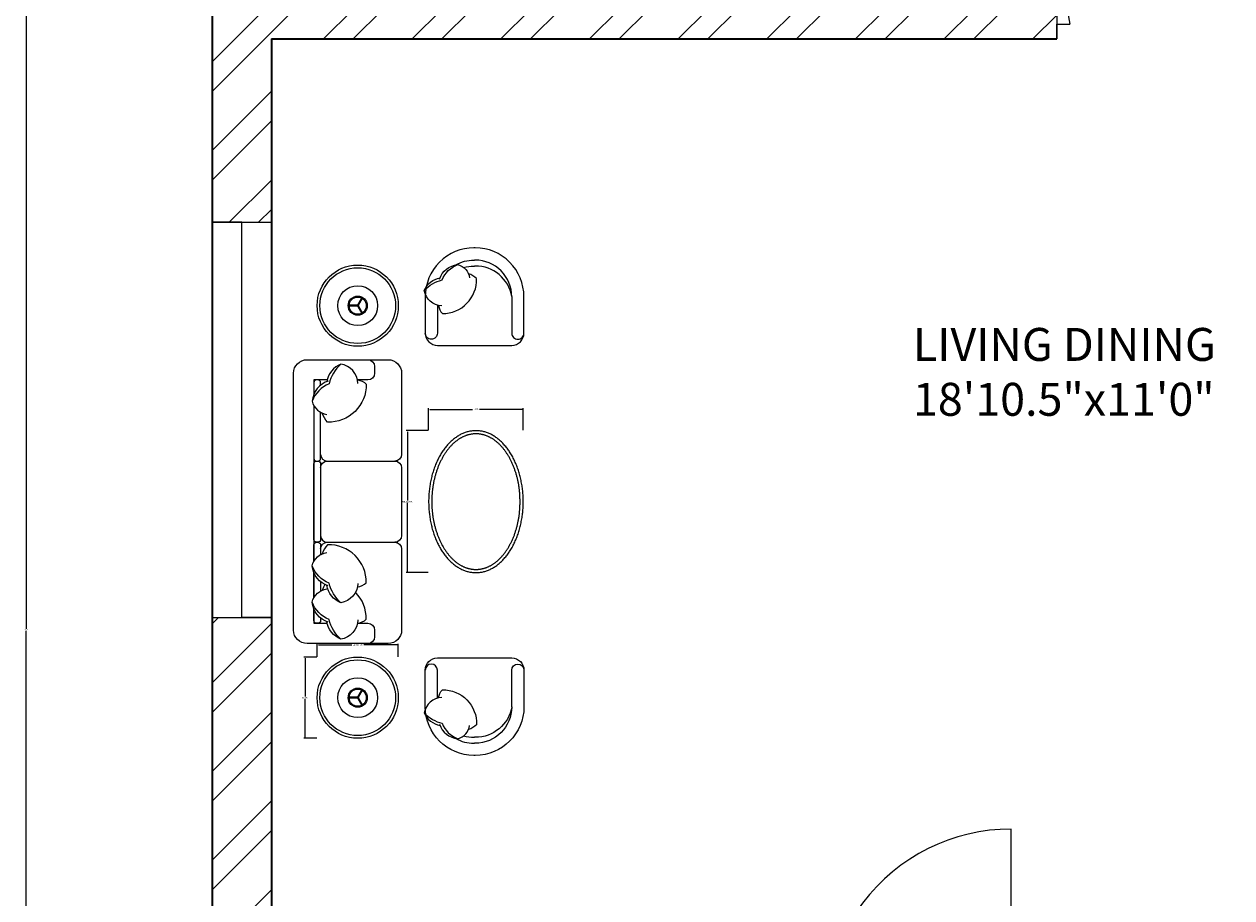
# Model space of a CAD drawing. Units: inches. Extents: x 1850 to 3445, y 1558 to 2756.
# Tile 2 of 13: x 2012 to 2195, y 1940 to 2073. Entities that reach past the tile are written whole.
import ezdxf

# ---------------------------------------------------------------- set-up
doc = ezdxf.new("R2010")
doc.units = ezdxf.units.IN
for name, color, linetype, lineweight in [('A-ANNO-DIMS', 2, 'Continuous', 18), ('A-AREA-IDEN', 7, 'Continuous', 18), ('A-DOOR', 3, 'Continuous', 18), ('A-FURN', 8, 'Continuous', 13), ('A-GLAZ', 4, 'Continuous', 18), ('A-WALL', 7, 'Continuous', 35), ('A-WALL-PATT', 252, 'Continuous', 13)]:
    doc.layers.add(name, color=color, linetype=linetype, lineweight=lineweight)
doc.styles.get("Standard").update_dxf_attribs({"font": 'arial.ttf'})
doc.dimstyles.get("Standard").update_dxf_attribs({"dimtxt": 0.18, "dimasz": 0.18, "dimexe": 0.18, "dimexo": 0.0625, "dimgap": 0.09, "dimtad": 0, "dimtih": 1, "dimtoh": 1, "dimdec": 4, "dimzin": 0, "dimdsep": 46, "dimtxsty": 'Standard', "dimcen": 0.09, "dimadec": 0, "dimazin": 0, "dimtfac": 1, "dimtdec": 4, "dimtofl": 0, "dimtmove": 0, "dimatfit": 3, "dimfxl": 1, "dimtolj": 1, "dimtzin": 0, "dimarcsym": 0})

# ---------------------------------------------------------------- blocks, each defined once
blk = doc.blocks.new('LAMP-ROUND-PLAN')
at = {"ltscale": 0.03}
for p, q in [((6.1, 6.13), (5.38, 7.38)), ((6.21, 6.19), (5.49, 7.44)), ((6.1, 6.19), (5.38, 4.94)), ((6.21, 6.13), (5.49, 4.87)), ((6.16, 6.22), (7.61, 6.22)), ((6.16, 6.09), (7.61, 6.09))]:
    blk.add_line(p, q, dxfattribs=at)
for radius in [6.16, 3.03, 1.45, 1.3]:
    blk.add_circle((6.16, 6.16), radius, dxfattribs=at)
blk.add_circle((6.16, 6.16), 5.75)
blk = doc.blocks.new('TABLE-COFFEE-OVAL')
at = {"ltscale": 0.03}
blk.add_polyline3d([(7.18, 0, 0), (7.32, 0, 0), (7.46, 0.01, 0), (7.59, 0.02, 0), (7.73, 0.03, 0), (7.86, 0.05, 0), (8, 0.07, 0), (8.13, 0.09, 0), (8.27, 0.12, 0), (8.4, 0.16, 0), (8.54, 0.19, 0), (8.67, 0.23, 0), (8.8, 0.28, 0), (8.93, 0.32, 0), (9.07, 0.38, 0), (9.2, 0.43, 0), (9.33, 0.49, 0), (9.46, 0.55, 0), (9.58, 0.62, 0), (9.71, 0.69, 0), (9.84, 0.76, 0), (9.96, 0.84, 0), (10.09, 0.92, 0), (10.21, 1.01, 0), (10.34, 1.09, 0), (10.46, 1.18, 0), (10.58, 1.28, 0), (10.7, 1.38, 0), (10.82, 1.48, 0), (10.93, 1.58, 0), (11.05, 1.69, 0), (11.16, 1.8, 0), (11.27, 1.92, 0), (11.38, 2.03, 0), (11.49, 2.16, 0), (11.6, 2.28, 0), (11.71, 2.41, 0), (11.81, 2.54, 0), (11.92, 2.67, 0), (12.02, 2.8, 0), (12.12, 2.94, 0), (12.22, 3.08, 0), (12.31, 3.23, 0), (12.41, 3.38, 0), (12.5, 3.53, 0), (12.59, 3.68, 0), (12.68, 3.83, 0), (12.76, 3.99, 0), (12.85, 4.15, 0), (12.93, 4.31, 0), (13.01, 4.48, 0), (13.09, 4.64, 0), (13.17, 4.81, 0), (13.24, 4.98, 0), (13.31, 5.15, 0), (13.38, 5.33, 0), (13.45, 5.51, 0), (13.52, 5.69, 0), (13.58, 5.87, 0), (13.64, 6.05, 0), (13.7, 6.23, 0), (13.75, 6.42, 0), (13.81, 6.61, 0), (13.86, 6.79, 0), (13.91, 6.98, 0), (13.96, 7.18, 0), (14, 7.37, 0), (14.04, 7.56, 0), (14.08, 7.76, 0), (14.12, 7.95, 0), (14.15, 8.15, 0), (14.18, 8.35, 0), (14.21, 8.55, 0), (14.24, 8.75, 0), (14.26, 8.95, 0), (14.29, 9.15, 0), (14.31, 9.35, 0), (14.32, 9.56, 0), (14.34, 9.76, 0), (14.35, 9.96, 0), (14.36, 10.17, 0), (14.36, 10.37, 0), (14.37, 10.57, 0), (14.37, 10.78, 0), (14.37, 10.98, 0), (14.36, 11.18, 0), (14.36, 11.39, 0), (14.35, 11.59, 0), (14.34, 11.8, 0), (14.32, 12, 0), (14.31, 12.2, 0), (14.29, 12.4, 0), (14.26, 12.6, 0), (14.24, 12.8, 0), (14.21, 13, 0), (14.18, 13.2, 0), (14.15, 13.4, 0), (14.12, 13.6, 0), (14.08, 13.8, 0), (14.04, 13.99, 0), (14, 14.18, 0), (13.96, 14.38, 0), (13.91, 14.57, 0), (13.86, 14.76, 0), (13.81, 14.95, 0), (13.75, 15.14, 0), (13.7, 15.32, 0), (13.64, 15.5, 0), (13.58, 15.69, 0), (13.52, 15.87, 0), (13.45, 16.05, 0), (13.38, 16.22, 0), (13.31, 16.4, 0), (13.24, 16.57, 0), (13.17, 16.74, 0), (13.09, 16.91, 0), (13.01, 17.08, 0), (12.93, 17.24, 0), (12.85, 17.4, 0), (12.76, 17.56, 0), (12.68, 17.72, 0), (12.59, 17.88, 0), (12.5, 18.03, 0), (12.41, 18.18, 0), (12.31, 18.32, 0), (12.22, 18.47, 0), (12.12, 18.61, 0), (12.02, 18.75, 0), (11.92, 18.88, 0), (11.81, 19.02, 0), (11.71, 19.15, 0), (11.6, 19.27, 0), (11.49, 19.4, 0), (11.38, 19.52, 0), (11.27, 19.64, 0), (11.16, 19.75, 0), (11.05, 19.86, 0), (10.93, 19.97, 0), (10.82, 20.08, 0), (10.7, 20.18, 0), (10.58, 20.27, 0), (10.46, 20.37, 0), (10.34, 20.46, 0), (10.21, 20.55, 0), (10.09, 20.63, 0), (9.96, 20.71, 0), (9.84, 20.79, 0), (9.71, 20.86, 0), (9.58, 20.93, 0), (9.46, 21, 0), (9.33, 21.06, 0), (9.2, 21.12, 0), (9.07, 21.18, 0), (8.93, 21.23, 0), (8.8, 21.28, 0), (8.67, 21.32, 0), (8.54, 21.36, 0), (8.4, 21.4, 0), (8.27, 21.43, 0), (8.13, 21.46, 0), (8, 21.48, 0), (7.86, 21.5, 0), (7.73, 21.52, 0), (7.59, 21.54, 0), (7.46, 21.55, 0), (7.32, 21.55, 0), (7.18, 21.55, 0), (7.05, 21.55, 0), (6.91, 21.55, 0), (6.78, 21.54, 0), (6.64, 21.52, 0), (6.5, 21.5, 0), (6.37, 21.48, 0), (6.23, 21.46, 0), (6.1, 21.43, 0), (5.97, 21.4, 0), (5.83, 21.36, 0), (5.7, 21.32, 0), (5.57, 21.28, 0), (5.43, 21.23, 0), (5.3, 21.18, 0), (5.17, 21.12, 0), (5.04, 21.06, 0), (4.91, 21, 0), (4.78, 20.93, 0), (4.66, 20.86, 0), (4.53, 20.79, 0), (4.4, 20.71, 0), (4.28, 20.63, 0), (4.15, 20.55, 0), (4.03, 20.46, 0), (3.91, 20.37, 0), (3.79, 20.27, 0), (3.67, 20.18, 0), (3.55, 20.08, 0), (3.44, 19.97, 0), (3.32, 19.86, 0), (3.21, 19.75, 0), (3.09, 19.64, 0), (2.98, 19.52, 0), (2.87, 19.4, 0), (2.77, 19.27, 0), (2.66, 19.15, 0), (2.55, 19.02, 0), (2.45, 18.88, 0), (2.35, 18.75, 0), (2.25, 18.61, 0), (2.15, 18.47, 0), (2.06, 18.32, 0), (1.96, 18.18, 0), (1.87, 18.03, 0), (1.78, 17.88, 0), (1.69, 17.72, 0), (1.6, 17.56, 0), (1.52, 17.4, 0), (1.44, 17.24, 0), (1.36, 17.08, 0), (1.28, 16.91, 0), (1.2, 16.74, 0), (1.13, 16.57, 0), (1.05, 16.4, 0), (0.98, 16.22, 0), (0.92, 16.05, 0), (0.85, 15.87, 0), (0.79, 15.69, 0), (0.73, 15.5, 0), (0.67, 15.32, 0), (0.61, 15.14, 0), (0.56, 14.95, 0), (0.51, 14.76, 0), (0.46, 14.57, 0), (0.41, 14.38, 0), (0.37, 14.18, 0), (0.33, 13.99, 0), (0.29, 13.8, 0), (0.25, 13.6, 0), (0.22, 13.4, 0), (0.18, 13.2, 0), (0.15, 13, 0), (0.13, 12.8, 0), (0.1, 12.6, 0), (0.08, 12.4, 0), (0.06, 12.2, 0), (0.05, 12, 0), (0.03, 11.8, 0), (0.02, 11.59, 0), (0.01, 11.39, 0), (0, 11.18, 0), (0, 10.98, 0), (0, 10.78, 0), (0, 10.57, 0), (0, 10.37, 0), (0.01, 10.17, 0), (0.02, 9.96, 0), (0.03, 9.76, 0), (0.05, 9.56, 0), (0.06, 9.35, 0), (0.08, 9.15, 0), (0.1, 8.95, 0), (0.13, 8.75, 0), (0.15, 8.55, 0), (0.18, 8.35, 0), (0.22, 8.15, 0), (0.25, 7.95, 0), (0.29, 7.76, 0), (0.33, 7.56, 0), (0.37, 7.37, 0), (0.41, 7.18, 0), (0.46, 6.98, 0), (0.51, 6.79, 0), (0.56, 6.61, 0), (0.61, 6.42, 0), (0.67, 6.23, 0), (0.73, 6.05, 0), (0.79, 5.87, 0), (0.85, 5.69, 0), (0.92, 5.51, 0), (0.98, 5.33, 0), (1.05, 5.15, 0), (1.13, 4.98, 0), (1.2, 4.81, 0), (1.28, 4.64, 0), (1.36, 4.48, 0), (1.44, 4.31, 0), (1.52, 4.15, 0), (1.6, 3.99, 0), (1.69, 3.83, 0), (1.78, 3.68, 0), (1.87, 3.53, 0), (1.96, 3.38, 0), (2.06, 3.23, 0), (2.15, 3.08, 0), (2.25, 2.94, 0), (2.35, 2.8, 0), (2.45, 2.67, 0), (2.55, 2.54, 0), (2.66, 2.41, 0), (2.77, 2.28, 0), (2.87, 2.16, 0), (2.98, 2.03, 0), (3.09, 1.92, 0), (3.21, 1.8, 0), (3.32, 1.69, 0), (3.44, 1.58, 0), (3.55, 1.48, 0), (3.67, 1.38, 0), (3.79, 1.28, 0), (3.91, 1.18, 0), (4.03, 1.09, 0), (4.15, 1.01, 0), (4.28, 0.92, 0), (4.4, 0.84, 0), (4.53, 0.76, 0), (4.66, 0.69, 0), (4.78, 0.62, 0), (4.91, 0.55, 0), (5.04, 0.49, 0), (5.17, 0.43, 0), (5.3, 0.38, 0), (5.43, 0.32, 0), (5.57, 0.28, 0), (5.7, 0.23, 0), (5.83, 0.19, 0), (5.97, 0.16, 0), (6.1, 0.12, 0), (6.23, 0.09, 0), (6.37, 0.07, 0), (6.5, 0.05, 0), (6.64, 0.03, 0), (6.78, 0.02, 0), (6.91, 0.01, 0), (7.05, 0, 0), (7.18, 0, 0)], dxfattribs=at)
blk.add_polyline3d([(7.18, 0.48, 0), (7.26, 0.48, 0), (7.33, 0.48, 0), (7.41, 0.49, 0), (7.48, 0.49, 0), (7.55, 0.5, 0), (7.63, 0.5, 0), (7.7, 0.51, 0), (7.78, 0.52, 0), (7.86, 0.53, 0), (7.93, 0.54, 0), (8.01, 0.56, 0), (8.09, 0.57, 0), (8.16, 0.59, 0), (8.24, 0.61, 0), (8.32, 0.63, 0), (8.39, 0.65, 0), (8.47, 0.67, 0), (8.55, 0.7, 0), (8.63, 0.72, 0), (8.71, 0.75, 0), (8.78, 0.78, 0), (8.86, 0.81, 0), (8.94, 0.84, 0), (9.02, 0.88, 0), (9.1, 0.91, 0), (9.18, 0.95, 0), (9.26, 0.99, 0), (9.33, 1.03, 0), (9.41, 1.07, 0), (9.49, 1.12, 0), (9.57, 1.16, 0), (9.65, 1.21, 0), (9.73, 1.26, 0), (9.8, 1.31, 0), (9.88, 1.36, 0), (9.96, 1.41, 0), (10.04, 1.47, 0), (10.11, 1.53, 0), (10.19, 1.58, 0), (10.27, 1.64, 0), (10.34, 1.71, 0), (10.42, 1.77, 0), (10.5, 1.84, 0), (10.57, 1.9, 0), (10.65, 1.97, 0), (10.72, 2.04, 0), (10.79, 2.12, 0), (10.87, 2.19, 0), (10.94, 2.27, 0), (11.01, 2.34, 0), (11.09, 2.42, 0), (11.16, 2.5, 0), (11.23, 2.58, 0), (11.3, 2.67, 0), (11.37, 2.75, 0), (11.44, 2.84, 0), (11.5, 2.93, 0), (11.57, 3.02, 0), (11.64, 3.11, 0), (11.71, 3.2, 0), (11.77, 3.3, 0), (11.84, 3.39, 0), (11.9, 3.49, 0), (11.96, 3.59, 0), (12.03, 3.68, 0), (12.09, 3.78, 0), (12.15, 3.89, 0), (12.21, 3.99, 0), (12.27, 4.09, 0), (12.33, 4.2, 0), (12.38, 4.3, 0), (12.44, 4.41, 0), (12.5, 4.52, 0), (12.55, 4.63, 0), (12.6, 4.74, 0), (12.66, 4.85, 0), (12.71, 4.96, 0), (12.76, 5.08, 0), (12.81, 5.19, 0), (12.86, 5.3, 0), (12.9, 5.42, 0), (12.95, 5.54, 0), (12.99, 5.65, 0), (13.04, 5.77, 0), (13.08, 5.89, 0), (13.12, 6.01, 0), (13.16, 6.13, 0), (13.2, 6.25, 0), (13.24, 6.37, 0), (13.28, 6.49, 0), (13.31, 6.61, 0), (13.35, 6.73, 0), (13.38, 6.85, 0), (13.41, 6.97, 0), (13.44, 7.09, 0), (13.47, 7.21, 0), (13.5, 7.34, 0), (13.53, 7.46, 0), (13.56, 7.58, 0), (13.58, 7.7, 0), (13.61, 7.83, 0), (13.63, 7.95, 0), (13.65, 8.07, 0), (13.68, 8.19, 0), (13.7, 8.32, 0), (13.72, 8.44, 0), (13.73, 8.56, 0), (13.75, 8.69, 0), (13.77, 8.81, 0), (13.78, 8.94, 0), (13.8, 9.06, 0), (13.81, 9.19, 0), (13.82, 9.31, 0), (13.83, 9.43, 0), (13.84, 9.56, 0), (13.85, 9.68, 0), (13.86, 9.81, 0), (13.87, 9.93, 0), (13.87, 10.06, 0), (13.88, 10.18, 0), (13.88, 10.31, 0), (13.89, 10.43, 0), (13.89, 10.56, 0), (13.89, 10.68, 0), (13.89, 10.81, 0), (13.89, 10.93, 0), (13.89, 11.06, 0), (13.88, 11.18, 0), (13.88, 11.31, 0), (13.88, 11.43, 0), (13.87, 11.56, 0), (13.86, 11.68, 0), (13.86, 11.81, 0), (13.85, 11.93, 0), (13.84, 12.06, 0), (13.83, 12.18, 0), (13.82, 12.31, 0), (13.8, 12.43, 0), (13.79, 12.55, 0), (13.77, 12.68, 0), (13.76, 12.8, 0), (13.74, 12.93, 0), (13.72, 13.05, 0), (13.71, 13.17, 0), (13.69, 13.3, 0), (13.66, 13.42, 0), (13.64, 13.54, 0), (13.62, 13.67, 0), (13.6, 13.79, 0), (13.57, 13.91, 0), (13.54, 14.03, 0), (13.52, 14.16, 0), (13.49, 14.28, 0), (13.46, 14.4, 0), (13.43, 14.52, 0), (13.4, 14.64, 0), (13.36, 14.76, 0), (13.33, 14.88, 0), (13.29, 15.01, 0), (13.26, 15.13, 0), (13.22, 15.25, 0), (13.18, 15.36, 0), (13.14, 15.48, 0), (13.1, 15.6, 0), (13.06, 15.72, 0), (13.02, 15.84, 0), (12.97, 15.96, 0), (12.93, 16.07, 0), (12.88, 16.19, 0), (12.83, 16.31, 0), (12.78, 16.42, 0), (12.73, 16.53, 0), (12.68, 16.65, 0), (12.63, 16.76, 0), (12.58, 16.87, 0), (12.52, 16.98, 0), (12.47, 17.09, 0), (12.41, 17.2, 0), (12.36, 17.3, 0), (12.3, 17.41, 0), (12.24, 17.51, 0), (12.18, 17.62, 0), (12.12, 17.72, 0), (12.06, 17.82, 0), (12, 17.92, 0), (11.93, 18.02, 0), (11.87, 18.11, 0), (11.8, 18.21, 0), (11.74, 18.3, 0), (11.67, 18.4, 0), (11.61, 18.49, 0), (11.54, 18.58, 0), (11.47, 18.67, 0), (11.4, 18.76, 0), (11.33, 18.84, 0), (11.26, 18.93, 0), (11.19, 19.01, 0), (11.12, 19.09, 0), (11.05, 19.17, 0), (10.98, 19.25, 0), (10.9, 19.33, 0), (10.83, 19.4, 0), (10.76, 19.47, 0), (10.68, 19.55, 0), (10.61, 19.62, 0), (10.53, 19.68, 0), (10.46, 19.75, 0), (10.38, 19.82, 0), (10.31, 19.88, 0), (10.23, 19.94, 0), (10.15, 20, 0), (10.08, 20.06, 0), (10, 20.11, 0), (9.92, 20.17, 0), (9.84, 20.22, 0), (9.77, 20.27, 0), (9.69, 20.32, 0), (9.61, 20.37, 0), (9.53, 20.42, 0), (9.45, 20.46, 0), (9.37, 20.5, 0), (9.3, 20.54, 0), (9.22, 20.58, 0), (9.14, 20.62, 0), (9.06, 20.66, 0), (8.98, 20.69, 0), (8.9, 20.73, 0), (8.82, 20.76, 0), (8.75, 20.79, 0), (8.67, 20.82, 0), (8.59, 20.84, 0), (8.51, 20.87, 0), (8.43, 20.89, 0), (8.36, 20.91, 0), (8.28, 20.93, 0), (8.2, 20.95, 0), (8.12, 20.97, 0), (8.05, 20.99, 0), (7.97, 21, 0), (7.89, 21.02, 0), (7.82, 21.03, 0), (7.74, 21.04, 0), (7.67, 21.05, 0), (7.59, 21.05, 0), (7.52, 21.06, 0), (7.44, 21.07, 0), (7.37, 21.07, 0), (7.29, 21.07, 0), (7.22, 21.07, 0), (7.15, 21.07, 0), (7.07, 21.07, 0), (7, 21.07, 0), (6.93, 21.07, 0), (6.85, 21.06, 0), (6.78, 21.05, 0), (6.7, 21.05, 0), (6.62, 21.04, 0), (6.55, 21.03, 0), (6.47, 21.02, 0), (6.4, 21, 0), (6.32, 20.99, 0), (6.24, 20.97, 0), (6.17, 20.95, 0), (6.09, 20.93, 0), (6.01, 20.91, 0), (5.93, 20.89, 0), (5.86, 20.87, 0), (5.78, 20.84, 0), (5.7, 20.82, 0), (5.62, 20.79, 0), (5.54, 20.76, 0), (5.47, 20.73, 0), (5.39, 20.69, 0), (5.31, 20.66, 0), (5.23, 20.62, 0), (5.15, 20.58, 0), (5.07, 20.54, 0), (4.99, 20.5, 0), (4.92, 20.46, 0), (4.84, 20.42, 0), (4.76, 20.37, 0), (4.68, 20.32, 0), (4.6, 20.27, 0), (4.52, 20.22, 0), (4.45, 20.17, 0), (4.37, 20.11, 0), (4.29, 20.06, 0), (4.21, 20, 0), (4.14, 19.94, 0), (4.06, 19.88, 0), (3.98, 19.82, 0), (3.91, 19.75, 0), (3.83, 19.68, 0), (3.76, 19.62, 0), (3.68, 19.55, 0), (3.61, 19.47, 0), (3.54, 19.4, 0), (3.46, 19.33, 0), (3.39, 19.25, 0), (3.32, 19.17, 0), (3.25, 19.09, 0), (3.18, 19.01, 0), (3.11, 18.93, 0), (3.04, 18.84, 0), (2.97, 18.76, 0), (2.9, 18.67, 0), (2.83, 18.58, 0), (2.76, 18.49, 0), (2.69, 18.4, 0), (2.63, 18.3, 0), (2.56, 18.21, 0), (2.5, 18.11, 0), (2.44, 18.02, 0), (2.37, 17.92, 0), (2.31, 17.82, 0), (2.25, 17.72, 0), (2.19, 17.62, 0), (2.13, 17.51, 0), (2.07, 17.41, 0), (2.01, 17.3, 0), (1.96, 17.2, 0), (1.9, 17.09, 0), (1.84, 16.98, 0), (1.79, 16.87, 0), (1.74, 16.76, 0), (1.69, 16.65, 0), (1.63, 16.53, 0), (1.58, 16.42, 0), (1.54, 16.31, 0), (1.49, 16.19, 0), (1.44, 16.07, 0), (1.4, 15.96, 0), (1.35, 15.84, 0), (1.31, 15.72, 0), (1.27, 15.6, 0), (1.23, 15.48, 0), (1.19, 15.36, 0), (1.15, 15.25, 0), (1.11, 15.13, 0), (1.07, 15.01, 0), (1.04, 14.88, 0), (1, 14.76, 0), (0.97, 14.64, 0), (0.94, 14.52, 0), (0.91, 14.4, 0), (0.88, 14.28, 0), (0.85, 14.16, 0), (0.82, 14.03, 0), (0.8, 13.91, 0), (0.77, 13.79, 0), (0.75, 13.67, 0), (0.72, 13.54, 0), (0.7, 13.42, 0), (0.68, 13.3, 0), (0.66, 13.17, 0), (0.64, 13.05, 0), (0.63, 12.93, 0), (0.61, 12.8, 0), (0.59, 12.68, 0), (0.58, 12.55, 0), (0.56, 12.43, 0), (0.55, 12.31, 0), (0.54, 12.18, 0), (0.53, 12.06, 0), (0.52, 11.93, 0), (0.51, 11.81, 0), (0.5, 11.68, 0), (0.5, 11.56, 0), (0.49, 11.43, 0), (0.49, 11.31, 0), (0.48, 11.18, 0), (0.48, 11.06, 0), (0.48, 10.93, 0), (0.48, 10.81, 0), (0.48, 10.68, 0), (0.48, 10.56, 0), (0.48, 10.43, 0), (0.49, 10.31, 0), (0.49, 10.18, 0), (0.49, 10.06, 0), (0.5, 9.93, 0), (0.51, 9.81, 0), (0.52, 9.68, 0), (0.52, 9.56, 0), (0.53, 9.43, 0), (0.55, 9.31, 0), (0.56, 9.19, 0), (0.57, 9.06, 0), (0.59, 8.94, 0), (0.6, 8.81, 0), (0.62, 8.69, 0), (0.63, 8.56, 0), (0.65, 8.44, 0), (0.67, 8.32, 0), (0.69, 8.19, 0), (0.71, 8.07, 0), (0.74, 7.95, 0), (0.76, 7.83, 0), (0.78, 7.7, 0), (0.81, 7.58, 0), (0.84, 7.46, 0), (0.86, 7.34, 0), (0.89, 7.21, 0), (0.92, 7.09, 0), (0.96, 6.97, 0), (0.99, 6.85, 0), (1.02, 6.73, 0), (1.06, 6.61, 0), (1.09, 6.49, 0), (1.13, 6.37, 0), (1.17, 6.25, 0), (1.21, 6.13, 0), (1.25, 6.01, 0), (1.29, 5.89, 0), (1.33, 5.77, 0), (1.37, 5.65, 0), (1.42, 5.54, 0), (1.46, 5.42, 0), (1.51, 5.3, 0), (1.56, 5.19, 0), (1.61, 5.08, 0), (1.66, 4.96, 0), (1.71, 4.85, 0), (1.76, 4.74, 0), (1.82, 4.63, 0), (1.87, 4.52, 0), (1.93, 4.41, 0), (1.98, 4.3, 0), (2.04, 4.2, 0), (2.1, 4.09, 0), (2.16, 3.99, 0), (2.22, 3.89, 0), (2.28, 3.78, 0), (2.34, 3.68, 0), (2.4, 3.59, 0), (2.47, 3.49, 0), (2.53, 3.39, 0), (2.6, 3.3, 0), (2.66, 3.2, 0), (2.73, 3.11, 0), (2.8, 3.02, 0), (2.86, 2.93, 0), (2.93, 2.84, 0), (3, 2.75, 0), (3.07, 2.67, 0), (3.14, 2.58, 0), (3.21, 2.5, 0), (3.28, 2.42, 0), (3.35, 2.34, 0), (3.43, 2.27, 0), (3.5, 2.19, 0), (3.57, 2.12, 0), (3.65, 2.04, 0), (3.72, 1.97, 0), (3.8, 1.9, 0), (3.87, 1.84, 0), (3.95, 1.77, 0), (4.02, 1.71, 0), (4.1, 1.64, 0), (4.18, 1.58, 0), (4.25, 1.53, 0), (4.33, 1.47, 0), (4.41, 1.41, 0), (4.48, 1.36, 0), (4.56, 1.31, 0), (4.64, 1.26, 0), (4.72, 1.21, 0), (4.8, 1.16, 0), (4.88, 1.12, 0), (4.95, 1.07, 0), (5.03, 1.03, 0), (5.11, 0.99, 0), (5.19, 0.95, 0), (5.27, 0.91, 0), (5.35, 0.88, 0), (5.43, 0.84, 0), (5.5, 0.81, 0), (5.58, 0.78, 0), (5.66, 0.75, 0), (5.74, 0.72, 0), (5.82, 0.7, 0), (5.9, 0.67, 0), (5.97, 0.65, 0), (6.05, 0.63, 0), (6.13, 0.61, 0), (6.21, 0.59, 0), (6.28, 0.57, 0), (6.36, 0.56, 0), (6.43, 0.54, 0), (6.51, 0.53, 0), (6.59, 0.52, 0), (6.66, 0.51, 0), (6.74, 0.5, 0), (6.81, 0.5, 0), (6.89, 0.49, 0), (6.96, 0.49, 0), (7.04, 0.48, 0), (7.11, 0.48, 0), (7.18, 0.48, 0)])
blk = doc.blocks.new('CHAIR-LOUNGE-CUSHION')
at = {"ltscale": 0.03}
blk.add_lwpolyline([(7.5, 0), (1.85, 0, -0.414214), (0, 1.85), (0, 7.4, -0.414214), (7.4, 14.81), (7.5, 14.81), (7.59, 14.81, -0.414214), (14.99, 7.4), (14.99, 1.85, -0.414214), (13.14, 0), (7.5, 0)], format="xyb", dxfattribs=at)
for points in [[(1.85, 7.4, -0.414214), (7.4, 12.95), (7.5, 12.95)], [(10.34, 12.22, 0.130591), (7.59, 12.95), (7.5, 12.95)], [(1.85, 7.4, -0.372719), (7.4, 12.03), (7.5, 12.03)], [(9.17, 11.83, 0.072384), (7.59, 12.03), (7.5, 12.03)], [(12.81, 10.05, 0.306663), (10.05, 12.26, 0.30633), (8.25, 10.25, -0.872847)], [(15.14, 8.34, 0.14773), (12.44, 9.93, 0.213343), (10.05, 12.26, 0.178662)], [(12.96, 6.06, -0.165541), (12.38, 4.84, -0.425989), (7.19, 10.14, -0.121523), (8.42, 10.87, 7.115464)], [(12.49, 6, 0.356772), (15.14, 8.34, 0.249542), (12.74, 10.26, -9.61688)], [(1.85, 7.4), (1.85, 1.85, -0.414214), (0.92, 0.93), (0.92, 0.93, -0.414214), (0, 1.85)], [(13.14, 6.11), (13.14, 1.85, 0.414214), (14.07, 0.93), (14.07, 0.93, 0.414214), (14.99, 1.85)]]:
    blk.add_lwpolyline(points, format="xyb")
blk = doc.blocks.new('WIN-60-W9')
for p, q in [((0, 9), (0, 0)), ((60, 4.5), (60, 9)), ((60, 9), (60, 0)), ((0, 0), (0, 4.5)), ((0, 4.5), (60, 4.5))]:
    blk.add_line(p, q)
blk = doc.blocks.new('DOOR-BED-GROUND')
for p, q in [((31.38, 2.25), (31.38, 38.25)), ((0, 4.5), (0, 0)), ((33.38, 4.5), (33.38, 0)), ((0, 0), (0, 2.25)), ((0, 2.25), (2, 2.25)), ((33.38, 2.25), (31.38, 2.25)), ((33.38, 0), (33.38, 2.25))]:
    blk.add_line(p, q)
blk.add_arc((31.38, 8.26), 29.99, 90, 191.5706)
blk = doc.blocks.new('DOOR-ENTRY-GROUND')
for p, q in [((29.19, 4.5), (29.19, 40.5)), ((0, 9), (0, 2.33)), ((31.19, 9), (31.19, 0)), ((0, 0), (0, 4.46)), ((0, 4.46), (2, 4.46)), ((31.19, 4.5), (29.19, 4.5)), ((31.19, 0), (31.19, 4.5)), ((0, 2.33), (0, 0))]:
    blk.add_line(p, q)
blk.add_arc((29.19, 12.22), 28.28, 90, 195.9327)
blk = doc.blocks.new('*D46')
at = {"layer": 'A-ANNO-DIMS', "color": 0, "lineweight": -2, "transparency": 16777216}
for p, q in [((2056.24, 1976.89), (2056.24, 1978.85)), ((2056.42, 1978.67), (2061.5, 1978.67)), ((2068.38, 1978.67), (2063.3, 1978.67)), ((2068.56, 1976.89), (2068.56, 1978.85))]:
    blk.add_line(p, q, dxfattribs=at)
at = {"layer": 'A-ANNO-DIMS', "color": 0, "transparency": 16777216}
for points in [[(2056.42, 1978.7), (2056.42, 1978.64), (2056.24, 1978.67)], [(2068.38, 1978.7), (2068.38, 1978.64), (2068.56, 1978.67)]]:
    blk.add_solid(points, dxfattribs=at)
at = {"layer": 'Defpoints', "color": 0, "transparency": 16777216}
for p in [(2056.24, 1978.67), (2056.24, 1976.83), (2068.56, 1976.83)]:
    blk.add_point(p, dxfattribs=at)
at = {"layer": 'A-ANNO-DIMS', "color": 0, "transparency": 16777216, "insert": (2062.4, 1978.67), "char_height": 0.18, "attachment_point": 5}
blk.add_mtext('\\A1;LAMP 12 TYP.', dxfattribs=at)
blk = doc.blocks.new('*D47')
at = {"layer": 'A-ANNO-DIMS', "color": 0, "lineweight": -2, "transparency": 16777216}
for p, q in [((2056.18, 1976.83), (2054.21, 1976.83)), ((2054.39, 1976.65), (2054.39, 1970.85)), ((2054.39, 1964.69), (2054.39, 1970.49)), ((2056.18, 1964.51), (2054.21, 1964.51))]:
    blk.add_line(p, q, dxfattribs=at)
at = {"layer": 'A-ANNO-DIMS', "color": 0, "transparency": 16777216}
for points in [[(2054.36, 1976.65), (2054.42, 1976.65), (2054.39, 1976.83)], [(2054.36, 1964.69), (2054.42, 1964.69), (2054.39, 1964.51)]]:
    blk.add_solid(points, dxfattribs=at)
at = {"layer": 'Defpoints', "color": 0, "transparency": 16777216}
for p in [(2056.24, 1976.83), (2054.39, 1964.51), (2056.24, 1964.51)]:
    blk.add_point(p, dxfattribs=at)
at = {"layer": 'A-ANNO-DIMS', "color": 0, "transparency": 16777216, "insert": (2054.39, 1970.67), "char_height": 0.18, "attachment_point": 5}
blk.add_mtext('\\A1;12 TYP.', dxfattribs=at)
blk = doc.blocks.new('*D52')
at = {"layer": 'A-ANNO-DIMS', "color": 0, "lineweight": -2, "transparency": 16777216}
for p, q in [((2073.11, 2011.21), (2069.76, 2011.21)), ((2069.94, 2011.03), (2069.94, 2000.61)), ((2069.94, 1989.83), (2069.94, 2000.25)), ((2073.11, 1989.65), (2069.76, 1989.65))]:
    blk.add_line(p, q, dxfattribs=at)
at = {"layer": 'A-ANNO-DIMS', "color": 0, "transparency": 16777216}
for points in [[(2069.91, 2011.03), (2069.97, 2011.03), (2069.94, 2011.21)], [(2069.91, 1989.83), (2069.97, 1989.83), (2069.94, 1989.65)]]:
    blk.add_solid(points, dxfattribs=at)
at = {"layer": 'Defpoints', "color": 0, "transparency": 16777216}
for p in [(2073.17, 2011.21), (2069.94, 1989.65), (2073.17, 1989.65)]:
    blk.add_point(p, dxfattribs=at)
at = {"layer": 'A-ANNO-DIMS', "color": 0, "transparency": 16777216, "insert": (2069.94, 2000.43), "char_height": 0.18, "attachment_point": 5}
blk.add_mtext('\\A1;TABLE 22 TYP.', dxfattribs=at)
blk = doc.blocks.new('*D53')
at = {"layer": 'A-ANNO-DIMS', "color": 0, "lineweight": -2, "transparency": 16777216}
for p, q in [((2073.17, 2011.27), (2073.17, 2014.62)), ((2073.35, 2014.44), (2079.84, 2014.44)), ((2087.36, 2014.44), (2080.88, 2014.44)), ((2087.54, 2011.27), (2087.54, 2014.62))]:
    blk.add_line(p, q, dxfattribs=at)
at = {"layer": 'A-ANNO-DIMS', "color": 0, "transparency": 16777216}
for points in [[(2073.35, 2014.47), (2073.35, 2014.41), (2073.17, 2014.44)], [(2087.36, 2014.47), (2087.36, 2014.41), (2087.54, 2014.44)]]:
    blk.add_solid(points, dxfattribs=at)
at = {"layer": 'Defpoints', "color": 0, "transparency": 16777216}
for p in [(2073.17, 2014.44), (2073.17, 2011.21), (2087.54, 2011.21)]:
    blk.add_point(p, dxfattribs=at)
at = {"layer": 'A-ANNO-DIMS', "color": 0, "transparency": 16777216, "insert": (2080.36, 2014.44), "char_height": 0.18, "attachment_point": 5}
blk.add_mtext('\\A1;14 TYP.', dxfattribs=at)
blk = doc.blocks.new('*D81')
at = {"layer": 'A-ANNO-DIMS', "color": 0, "lineweight": -2, "transparency": 16777216}
for p, q in [((2040.21, 2216.18), (2011.84, 2216.18)), ((2012.02, 2216), (2012.02, 1981.12)), ((2012.02, 1745.86), (2012.02, 1980.75)), ((2040.21, 1745.68), (2011.84, 1745.68))]:
    blk.add_line(p, q, dxfattribs=at)
at = {"layer": 'A-ANNO-DIMS', "color": 0, "transparency": 16777216}
for points in [[(2011.99, 2216), (2012.05, 2216), (2012.02, 2216.18)], [(2011.99, 1745.86), (2012.05, 1745.86), (2012.02, 1745.68)]]:
    blk.add_solid(points, dxfattribs=at)
at = {"layer": 'Defpoints', "color": 0, "transparency": 16777216}
for p in [(2012.02, 2216.18), (2040.27, 2216.18), (2040.27, 1745.68)]:
    blk.add_point(p, dxfattribs=at)
at = {"layer": 'A-ANNO-DIMS', "color": 0, "transparency": 16777216, "insert": (2012.02, 1980.93), "char_height": 0.18, "attachment_point": 5}
blk.add_mtext('\\A1;470.5', dxfattribs=at)

msp = doc.modelspace()

# ---------------------------------------------------------------- hatches: boundary and pattern name
at = {"layer": 'A-WALL-PATT'}
h = msp.add_hatch(dxfattribs=at)
h.set_pattern_fill('ANSI32', color=256)
h.paths.add_polyline_path([(2519.5556, 1907.3936), (2523.9987, 1907.3936), (2523.9987, 1916.3936), (2519.5556, 1916.3936), (2515.0556, 1916.3936), (2510.5556, 1916.3936), (2510.5556, 1907.3936), (2515.0556, 1907.3936), (2515.0556, 1742.1843), (2515.0556, 1737.6843), (2596.0556, 1737.6843), (2596.0556, 1976.4962), (2591.5556, 1976.4962), (2591.5556, 1916.3936), (2561.2666, 1916.3936), (2561.2666, 1907.3936), (2591.5556, 1907.3936), (2591.5556, 1746.6843), (2519.5556, 1746.6843)])
h.paths.add_polyline_path([(2076.6481, 2211.6843), (2076.6481, 2216.1843), (2040.2715, 2216.1843), (2040.2715, 2175.83), (2044.7715, 2175.83), (2049.2715, 2175.83), (2049.2715, 2207.1843), (2076.6481, 2207.1843)])
h.paths.add_polyline_path([(2211.7715, 2216.1843), (2136.6481, 2216.1843), (2136.6481, 2207.1843), (2211.7715, 2207.1843)])
h.paths.add_polyline_path([(2285.2715, 2154.1843), (2250.6169, 2154.1843), (2250.6169, 2149.6843), (2280.7715, 2149.6843), (2280.7715, 2075.1843), (2236.3632, 2075.1843), (2236.3632, 2070.6843), (2285.2715, 2070.6843)])
h.paths.add_polyline_path([(2228.3485, 2154.1843), (2207.2715, 2154.1843), (2207.2715, 2075.1843), (2201.9819, 2075.1843), (2201.9819, 2070.6843), (2215.4663, 2070.6843), (2215.4663, 2072.9343), (2215.4663, 2075.1843), (2211.7715, 2075.1843), (2211.7715, 2149.6843), (2228.3485, 2149.6843)])
h.paths.add_polyline_path([(2049.2715, 2115.83), (2040.2715, 2115.83), (2040.2715, 2042.8465), (2049.2715, 2042.8465), (2049.2715, 2070.6843), (2168.6057, 2070.6843), (2168.6057, 2072.9343), (2168.6057, 2075.1843), (2049.2715, 2075.1843)])
h.paths.add_polyline_path([(2049.2715, 1982.8465), (2040.2715, 1982.8465), (2040.2715, 1910.2175), (2060.9481, 1910.2175), (2060.9481, 1914.7175), (2060.9481, 1919.2175), (2049.2715, 1919.2175)])
h.paths.add_polyline_path([(2132.4938, 1919.2175), (2108.9481, 1919.2175), (2108.9481, 1910.2175), (2132.4938, 1910.2175), (2132.4938, 1914.6749)])
h.paths.add_polyline_path([(2178.7715, 1938.6843), (2169.7715, 1938.6843), (2169.7715, 1919.2175), (2163.687, 1919.2175), (2163.687, 1910.2175), (2169.7715, 1910.2175), (2169.7715, 1854.6843), (2169.7715, 1845.6843), (2196.1287, 1845.6843), (2196.1287, 1850.1843), (2196.1287, 1854.6843), (2178.7715, 1854.6843)])
h.paths.add_polyline_path([(2049.2715, 1910.2175), (2040.2715, 1910.2175), (2040.2715, 1745.6843), (2049.2715, 1745.6843)])
h.paths.add_polyline_path([(2146.8861, 1766.7204), (2159.0894, 1766.7204), (2159.0894, 1777.0239), (2146.8861, 1777.0239)], flags=9)
h.paths.add_polyline_path([(2183.4664, 1798.4016), (2226.7338, 1798.4016), (2226.7338, 1817.0589), (2183.4664, 1817.0589)], flags=9)
h.paths.add_polyline_path([(2070.863, 1867.537), (2109.9796, 1867.537), (2109.9796, 1886.1943), (2070.863, 1886.1943)], flags=9)

# ---------------------------------------------------------------- linework, layer by layer
at = {"layer": 'A-FURN', "ltscale": 0.03}
msp.add_lwpolyline([(2067.0162, 2021.9834, -0.41421356), (2069.0688, 2019.9307), (2069.0688, 2007.6149, -0.41421356), (2068.0425, 2006.5886, -0.41421356), (2069.0688, 2005.5622), (2069.0688, 1995.299, -0.41421356), (2068.0425, 1994.2727, -0.41421356), (2069.0688, 1993.2464), (2069.0688, 1980.9305, -0.41421356), (2067.0162, 1978.8779), (2054.7003, 1978.8779, -0.41421356), (2052.6477, 1980.9305), (2052.6477, 2019.9307, -0.41421356), (2054.7003, 2021.9834)], format="xyb", close=True, dxfattribs=at)
at = {"layer": 'A-FURN'}
for points in [[(2059.8222, 2021.3302, 0.14772988), (2058.0584, 2018.3306, 0.21334276), (2055.4714, 2015.6838, 0.17866181)], [(2062.4092, 2018.3894, 0.35677236), (2059.8222, 2021.3302, 0.24954205), (2057.6904, 2018.6655, -9.61688035)], [(2063.9372, 2021.9834, -0.41421356), (2064.9635, 2020.9571), (2064.9635, 2019.9307, -0.41421356), (2063.9372, 2018.9044), (2062.3471, 2018.9044)], [(2057.9178, 2018.745, 0.30666349), (2055.4714, 2015.6838, 0.30632997), (2057.7056, 2013.684, -0.87284716)], [(2056.753, 2018.1212), (2056.753, 2018.4939, 0.41421356), (2056.3424, 2018.9044), (2056.1372, 2018.9044, 0.41421356), (2055.7266, 2018.4939)], [(2055.7266, 2018.4939), (2055.7266, 2016.7453, 0.41421356)], [(2062.3466, 2018.9067, -0.16554063), (2063.7027, 2018.2717, -0.42598917), (2057.8232, 2012.5077, -0.12152332), (2057.0128, 2013.876, 7.11546429)], [(2055.7266, 2015.0379), (2055.7266, 2006.9991, 0.41421356), (2056.1372, 2006.5886), (2056.3424, 2006.5886, 0.41421356), (2056.753, 2006.9991), (2056.753, 2014.0045, 0.41421356)], [(2056.753, 2007.6149, 0.41421356), (2057.7793, 2006.5886), (2068.0425, 2006.5886, 0.41421356)], [(2056.753, 2005.5622, -0.41421356), (2057.7793, 2006.5886)], [(2056.753, 1995.299, 0.41421356), (2057.7793, 1994.2727)], [(2055.7266, 1991.3521), (2055.7266, 1993.8622, -0.41421356), (2056.1372, 1994.2727), (2056.3424, 1994.2727, -0.41421356), (2056.753, 1993.8622), (2056.753, 1992.3856, -0.41421356)], [(2056.753, 1993.2464, -0.41421356), (2057.7793, 1994.2727), (2068.0425, 1994.2727, -0.41421356)], [(2062.3466, 1987.4833, 0.16554063), (2063.7027, 1988.1183, 0.42598917), (2057.8232, 1993.8823, 0.12152332), (2057.0128, 1992.514, -7.11546429)], [(2057.9178, 1987.645, -0.30666349), (2055.4714, 1990.7062, -0.30632997), (2057.7056, 1992.706, 0.87284716)], [(2059.8222, 1985.0598, -0.14772988), (2058.0584, 1988.0594, -0.21334276), (2055.4714, 1990.7062, -0.17866181)], [(2055.7266, 1985.8233), (2055.7266, 1989.6447, -0.41421356)], [(2056.753, 1988.2688), (2056.753, 1986.8568, -0.41421356)], [(2057.4141, 1987.8457, 0.07186538), (2057.0128, 1986.9853, -7.11546429)], [(2062.4092, 1988.0006, -0.35677236), (2059.8222, 1985.0598, -0.24954205), (2057.6904, 1987.7245, 9.61688035)], [(2057.9178, 1982.1163, -0.30666349), (2055.4714, 1985.1774, -0.30632997), (2057.7056, 1987.1772, 0.87284716)], [(2062.3466, 1981.9546, 0.16554063), (2063.7027, 1982.5895, 0.20023115), (2062.0511, 1986.6636, 0.12152332)], [(2059.8222, 1979.531, -0.14772988), (2058.0584, 1982.5307, -0.21334276), (2055.4714, 1985.1774, -0.17866181)], [(2055.7266, 1984.1159), (2055.7266, 1981.9568), (2057.7436, 1981.9568, -0.41421356)], [(2055.7266, 1982.3674), (2055.7266, 1984.1159, -0.41421356)], [(2056.753, 1982.74), (2056.753, 1982.3674, -0.41421356), (2056.3424, 1981.9568), (2056.1372, 1981.9568, -0.41421356), (2055.7266, 1982.3674)], [(2062.4092, 1982.4719, -0.35677236), (2059.8222, 1979.531, -0.24954205), (2057.6904, 1982.1957, 9.61688035)], [(2062.3471, 1981.9568), (2063.9372, 1981.9568, -0.41421356), (2064.9635, 1980.9305), (2064.9635, 1979.9042, -0.41421356), (2063.9372, 1978.8779)], [(2074.5083, 1970.5952), (2074.5083, 1974.85, 0.41421356), (2073.583, 1975.7754), (2073.583, 1975.7754, 0.41421356), (2072.6576, 1974.85)], [(2085.7979, 1969.2977), (2085.7979, 1974.85, -0.41421356), (2086.7233, 1975.7754), (2086.7233, 1975.7754, -0.41421356), (2087.6486, 1974.85)], [(2074.6914, 1970.6397, -0.16554063), (2075.2639, 1971.8624, -0.42598917), (2080.4609, 1966.5613, -0.12152332), (2079.2273, 1965.8306, 7.11546429)], [(2075.1578, 1970.6962, 0.35677236), (2072.5062, 1968.3636, 0.24954205), (2074.9088, 1966.4415, -9.61688035)], [(2085.7979, 1969.2978, -0.37271891), (2080.2457, 1964.6709), (2080.1531, 1964.6709)], [(2085.7979, 1969.2978, -0.41421356), (2080.2457, 1963.7455), (2080.1531, 1963.7455)], [(2072.5062, 1968.3636, 0.14772988), (2075.2108, 1966.7733, 0.21334276), (2077.5972, 1964.4408, 0.17866181)], [(2074.8372, 1966.6466, 0.30666349), (2077.5972, 1964.4408, 0.30632997), (2079.4003, 1966.4552, -0.87284716)], [(2077.3045, 1964.4779, 0.13059149), (2080.0606, 1963.7455), (2080.1531, 1963.7455)], [(2078.4829, 1964.8703, 0.07238424), (2080.0606, 1964.6709), (2080.1531, 1964.6709)]]:
    msp.add_lwpolyline(points, format="xyb", dxfattribs=at)
for points in [[(2057.7436, 2018.9044), (2055.7266, 2018.9044), (2055.7266, 2016.7453)], [(2055.7266, 2015.0379), (2055.7266, 1991.3521)], [(2055.7266, 1989.6447), (2055.7266, 1985.8233)]]:
    msp.add_lwpolyline(points, dxfattribs=at)
msp.add_lwpolyline([(2055.7266, 1994.6832), (2055.7266, 2006.178, -0.41421356), (2056.1372, 2006.5886), (2056.3424, 2006.5886, -0.41421356), (2056.753, 2006.178), (2056.753, 1994.6832, -0.41421356), (2056.3424, 1994.2727), (2056.1372, 1994.2727, -0.41421356)], format="xyb", close=True, dxfattribs=at)
at = {"layer": 'A-FURN', "ltscale": 0.03}
msp.add_lwpolyline([(2080.1531, 1976.7008), (2085.7979, 1976.7008, -0.41421356), (2087.6486, 1974.85), (2087.6486, 1969.2978, -0.41421356), (2080.2457, 1961.8948), (2080.1531, 1961.8948), (2080.0606, 1961.8948, -0.41421356), (2072.6576, 1969.2978), (2072.6576, 1974.85, -0.41421356), (2074.5083, 1976.7008), (2080.1531, 1976.7008)], format="xyb", dxfattribs=at)
at = {"layer": 'A-WALL'}
for p, q in [((2040.2715, 2216.1843), (2040.2715, 1745.6843)), ((2049.2715, 2070.6843), (2168.6057, 2070.6843)), ((2049.2715, 2070.6843), (2049.2715, 1919.2175))]:
    msp.add_line(p, q, dxfattribs=at)

# ---------------------------------------------------------------- block references
at = {"layer": 'A-DOOR'}
for name, p in [('DOOR-BED-GROUND', (2168.606, 2070.684)), ('DOOR-ENTRY-GROUND', (2132.494, 1910.217))]:
    msp.add_blockref(name, p, dxfattribs=at)
at = {"layer": 'A-FURN', "extrusion": (0, 0, -1), "zscale": -1}
msp.add_blockref('CHAIR-LOUNGE-CUSHION', (-2087.6481, 2024.1608), dxfattribs=at)
at = {"layer": 'A-FURN', "rotation": 180}
for name, p in [('LAMP-ROUND-PLAN', (2068.5561, 2036.3514)), ('TABLE-COFFEE-OVAL', (2087.5421, 2011.2074)), ('LAMP-ROUND-PLAN', (2068.5561, 1976.8247))]:
    msp.add_blockref(name, p, dxfattribs=at)
at = {"layer": 'A-GLAZ', "rotation": 90}
msp.add_blockref('WIN-60-W9', (2049.2718, 1982.8465), dxfattribs=at)

# ---------------------------------------------------------------- texts
at = {"layer": 'A-AREA-IDEN', "insert": (2146.752, 2026.8071), "char_height": 5, "attachment_point": 1}
msp.add_mtext_dynamic_manual_height_columns('LIVING DINING\\P18\'10.5"x11\'0"', width=127.083129, gutter_width=12.5, heights=[0], dxfattribs=at)

# ---------------------------------------------------------------- dimensions: what is measured, and where the dimension line sits
at = {"layer": 'A-ANNO-DIMS'}
dim = msp.add_linear_dim(base=(2012.0215, 2216.1843), p1=(2040.2715, 1745.6843), p2=(2040.2715, 2216.1843), angle=90, dimstyle='Standard', override={"dimdec": 1, "dimlfac": 1, "dimrnd": 0, "dimzin": 0, "dimdsep": 46, "dimlunit": 2}, dxfattribs=at)
dim.commit()
dim.dimension.update_dxf_attribs({"geometry": '*D81', "text_midpoint": (2012.0215, 1980.9343)})
for base, p1, p2, angle, text, picture, middle in [((2073.1741, 2014.4399), (2087.5426, 2011.207), (2073.1741, 2011.207), 180, '<> TYP.', '*D53', (2080.3584, 2014.4399)), ((2069.9412, 1989.6542), (2073.1741, 2011.207), (2073.1741, 1989.6542), 270, 'TABLE <> TYP.', '*D52', (2069.9412, 2000.4306)), ((2056.2398, 1978.6726), (2068.5557, 1976.8252), (2056.2398, 1976.8252), 180, 'LAMP <> TYP.', '*D46', (2062.3977, 1978.6726)), ((2054.3924, 1964.5093), (2056.2398, 1976.8252), (2056.2398, 1964.5093), 270, '<> TYP.', '*D47', (2054.3924, 1970.6673))]:
    dim = msp.add_linear_dim(base=base, p1=p1, p2=p2, angle=angle, text=text, dimstyle='Standard', override={"dimdec": 0, "dimlfac": 1, "dimrnd": 0, "dimzin": 0, "dimdsep": 46, "dimlunit": 2}, dxfattribs=at)
    dim.commit()
    dim.dimension.update_dxf_attribs({"geometry": picture, "text_midpoint": middle})

doc.saveas('drawing.dxf')
